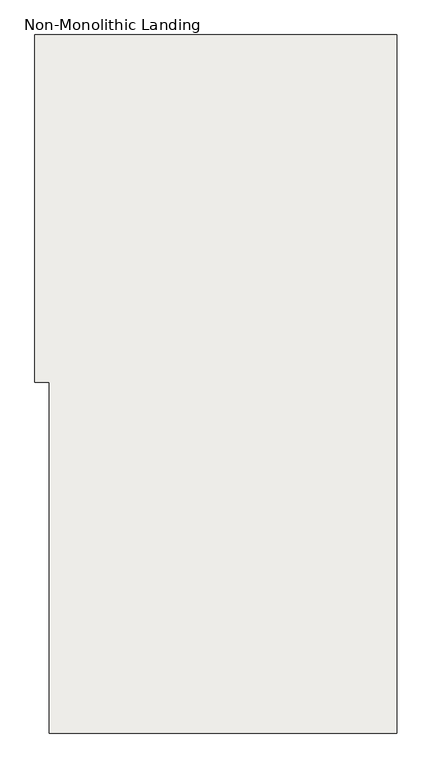
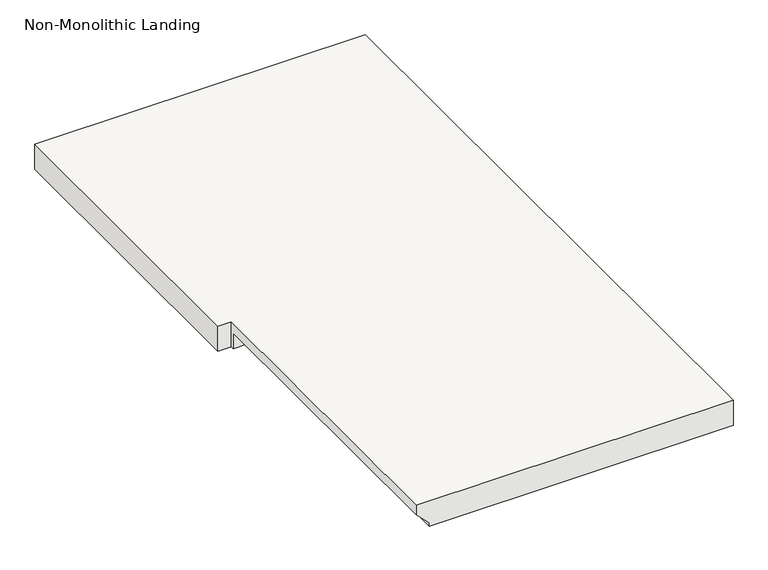
"""IFC4 building model written with IfcOpenShell, lengths in millimetres: slab geometry, Non-Monolithic Landing."""

from ifc_helpers import new_model, si_unit, origin, place, context, project, spatial, faceted_brep, source, transform, mapped, element, save


def non_monolithic_landing_e6237f85(model_context):
    return source(origin(), model_context, "Body", "Brep", [
        faceted_brep([(-2686.4237097, 3724.9480625, 1600.2), (-2686.4237097, 4950.7083475, 1600.2), (-3296.0237097, 4950.7083475, 1600.2), (-3321.4237097, 4950.7083475, 1600.2), (-3321.4237097, 4341.1083475, 1600.2), (-3296.0237097, 4341.1083475, 1600.2), (-3296.0237097, 3724.9480625, 1600.2), (-3270.6237097, 4334.5480625, 1549.4), (-3296.0237097, 4334.5480625, 1549.4), (-3296.0237097, 4341.1083475, 1549.4), (-3321.4237097, 4341.1083475, 1549.4), (-3321.4237097, 4950.7083475, 1549.4), (-3296.0237097, 4950.7083475, 1549.4), (-2686.4237097, 4950.7083475, 1549.4), (-2686.4237097, 3724.9480625, 1549.4), (-3270.6237097, 3724.9480625, 1549.4), (-3296.0237097, 4334.5480625, 1581.15), (-3296.0237097, 3724.9480625, 1581.15), (-3270.6237097, 3724.9480625, 1555.75), (-3270.6237097, 4334.5480625, 1555.75)], [[[0, 1, 2, 3, 4, 5, 6]], [[7, 8, 9, 10, 11, 12, 13, 14, 15]], [[2, 1, 13, 12]], [[4, 3, 11, 10]], [[3, 2, 12, 11]], [[6, 5, 9, 8, 16, 17]], [[0, 6, 17, 18, 15, 14]], [[18, 17, 16, 19]], [[8, 7, 19, 16]], [[7, 15, 18, 19]], [[1, 0, 14, 13]], [[5, 4, 10, 9]]]),
    ])


if __name__ == "__main__":
    model = new_model("IFC4")
    model_context = context("Model", 3, world=origin())
    ifc_project = project(units=[si_unit("LENGTHUNIT", "METRE", prefix="MILLI")], contexts=[model_context])
    site = spatial("IfcSite", under=ifc_project)
    building = spatial("IfcBuilding", under=site)
    placement = place(None, origin())
    non_monolithic_landing_shape = non_monolithic_landing_e6237f85(model_context)
    element("IfcSlab", 1, ObjectType="Non-Monolithic Landing", at=placement, inside=building, context=model_context, shape_type="MappedRepresentation", body=[
        mapped(non_monolithic_landing_shape, transform((0.0, 0.0, 0.0), x_axis=(1.0, 0.0, 0.0), y_axis=(0.0, 1.0, 0.0), z_axis=(0.0, 0.0, 1.0))),
    ])
    save(model, "model.ifc")
